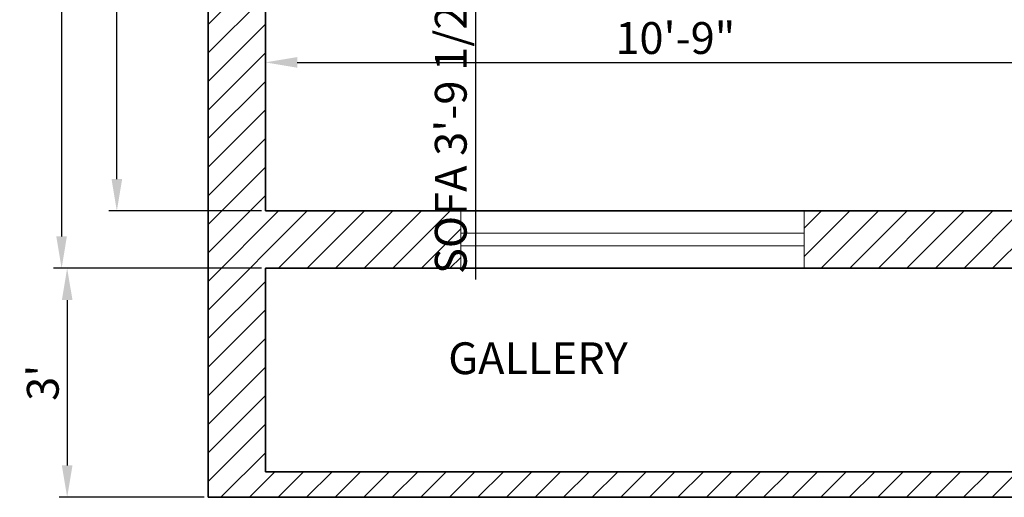
# Model space of a CAD drawing. Units: inches. Extents: x -33 to 381, y -443 to 47.
# Tile 1 of 5: x -33 to 122, y -383 to -308. Entities that reach past the tile are written whole.
import ezdxf

# ---------------------------------------------------------------- set-up
doc = ezdxf.new("R2010")
doc.units = ezdxf.units.IN
for name, color, linetype, lineweight in [('A-ANNO-DIMS', 2, 'Continuous', 18), ('A-AREA-IDEN', 7, 'Continuous', 18), ('A-GLAZ', 4, 'Continuous', 18), ('A-WALL', 7, 'Continuous', 35), ('A-WALL-PATT', 251, 'Continuous', 13)]:
    doc.layers.add(name, color=color, linetype=linetype, lineweight=lineweight)
doc.styles.get("Standard").update_dxf_attribs({"font": 'arial.ttf'})
doc.dimstyles.new('ISO-25', dxfattribs={"dimtxt": 5, "dimasz": 5, "dimexe": 1.25, "dimexo": 0.625, "dimtad": 1, "dimlunit": 3, "dimtxsty": 'Standard', "dimcen": 2.5, "dimadec": 0, "dimazin": 0, "dimtfac": 1, "dimtmove": 0, "dimatfit": 3, "dimfxl": 1, "dimarcsym": 0})
pattern_1 = [(45, (-607.8963, -64.2963), (-2.245064, 2.245064), [])]

# ---------------------------------------------------------------- blocks, each defined once
blk = doc.blocks.new('*D11')
at = {"layer": 'A-ANNO-DIMS', "color": 0, "lineweight": -2, "transparency": 16777216}
for p, q in [((-4.08, 13.18), (-27.74, 13.18)), ((-26.49, 8.18), (-26.49, -341.82)), ((4.92, -346.82), (-27.74, -346.82))]:
    blk.add_line(p, q, dxfattribs=at)
at = {"layer": 'A-ANNO-DIMS', "color": 0, "transparency": 16777216}
for points in [[(-27.33, 8.18), (-25.66, 8.18), (-26.49, 13.18)], [(-27.33, -341.82), (-25.66, -341.82), (-26.49, -346.82)]]:
    blk.add_solid(points, dxfattribs=at)
at = {"layer": 'Defpoints', "color": 0, "transparency": 16777216}
for p in [(-3.46, 13.18), (-26.49, -346.82), (5.54, -346.82)]:
    blk.add_point(p, dxfattribs=at)
at = {"layer": 'A-ANNO-DIMS', "color": 0, "transparency": 16777216, "insert": (-29.67, -166.82), "char_height": 5, "attachment_point": 5, "rotation": 90}
blk.add_mtext("30'", dxfattribs=at)
blk = doc.blocks.new('*D12')
at = {"layer": 'A-ANNO-DIMS', "color": 0, "lineweight": -2, "transparency": 16777216}
for p, q in [((-4.08, -346.82), (-26.87, -346.82)), ((-25.62, -351.82), (-25.62, -377.82)), ((-4.08, -382.82), (-26.87, -382.82))]:
    blk.add_line(p, q, dxfattribs=at)
at = {"layer": 'A-ANNO-DIMS', "color": 0, "transparency": 16777216}
for points in [[(-26.45, -351.82), (-24.78, -351.82), (-25.62, -346.82)], [(-26.45, -377.82), (-24.78, -377.82), (-25.62, -382.82)]]:
    blk.add_solid(points, dxfattribs=at)
at = {"layer": 'Defpoints', "color": 0, "transparency": 16777216}
for p in [(-3.46, -346.82), (-25.62, -382.82), (-3.46, -382.82)]:
    blk.add_point(p, dxfattribs=at)
at = {"layer": 'A-ANNO-DIMS', "color": 0, "transparency": 16777216, "insert": (-28.8, -364.82), "char_height": 5, "attachment_point": 5, "rotation": 90}
blk.add_mtext("3'", dxfattribs=at)
blk = doc.blocks.new('*D21')
at = {"layer": 'A-ANNO-DIMS', "color": 0, "lineweight": -2, "transparency": 16777216}
for p, q in [((32.37, -251.08), (39.8, -251.08)), ((38.55, -256.08), (38.55, -291.45)), ((32.37, -296.45), (39.8, -296.45)), ((38.55, -296.45), (38.55, -348.58))]:
    blk.add_line(p, q, dxfattribs=at)
at = {"layer": 'A-ANNO-DIMS', "color": 0, "transparency": 16777216}
for points in [[(37.71, -256.08), (39.38, -256.08), (38.55, -251.08)], [(37.71, -291.45), (39.38, -291.45), (38.55, -296.45)]]:
    blk.add_solid(points, dxfattribs=at)
at = {"layer": 'Defpoints', "color": 0, "transparency": 16777216}
for p in [(31.74, -251.08), (31.74, -296.45), (38.55, -296.45)]:
    blk.add_point(p, dxfattribs=at)
at = {"layer": 'A-ANNO-DIMS', "color": 0, "transparency": 16777216, "insert": (35.33, -325.02), "char_height": 5, "attachment_point": 5, "rotation": 90}
blk.add_mtext('SOFA 3\'-9 1/2"', dxfattribs=at)
blk = doc.blocks.new('*D45')
at = {"layer": 'A-ANNO-DIMS', "color": 0, "lineweight": -2, "transparency": 16777216}
for p, q in [((4.92, -218.82), (-19.06, -218.82)), ((-17.81, -332.82), (-17.81, -223.82)), ((4.92, -337.82), (-19.06, -337.82))]:
    blk.add_line(p, q, dxfattribs=at)
at = {"layer": 'A-ANNO-DIMS', "color": 0, "transparency": 16777216}
for points in [[(-18.64, -223.82), (-16.98, -223.82), (-17.81, -218.82)], [(-18.64, -332.82), (-16.98, -332.82), (-17.81, -337.82)]]:
    blk.add_solid(points, dxfattribs=at)
at = {"layer": 'Defpoints', "color": 0, "transparency": 16777216}
for p in [(-17.81, -218.82), (5.54, -218.82), (5.54, -337.82)]:
    blk.add_point(p, dxfattribs=at)
at = {"layer": 'A-ANNO-DIMS', "color": 0, "transparency": 16777216, "insert": (-20.99, -278.32), "char_height": 5, "attachment_point": 5, "rotation": 90}
blk.add_mtext('9\'-11"', dxfattribs=at)
blk = doc.blocks.new('*D63')
at = {"layer": 'A-ANNO-DIMS', "color": 0, "lineweight": -2, "transparency": 16777216}
for p, q in [((5.54, -337.2), (5.54, -313.22)), ((134.42, -337.2), (134.42, -313.22)), ((10.54, -314.47), (129.42, -314.47))]:
    blk.add_line(p, q, dxfattribs=at)
at = {"layer": 'A-ANNO-DIMS', "color": 0, "transparency": 16777216}
for points in [[(10.54, -313.64), (10.54, -315.3), (5.54, -314.47)], [(129.42, -313.64), (129.42, -315.3), (134.42, -314.47)]]:
    blk.add_solid(points, dxfattribs=at)
at = {"layer": 'Defpoints', "color": 0, "transparency": 16777216}
for p in [(134.42, -314.47), (5.54, -337.82), (134.42, -337.82)]:
    blk.add_point(p, dxfattribs=at)
at = {"layer": 'A-ANNO-DIMS', "color": 0, "transparency": 16777216, "insert": (69.98, -311.29), "char_height": 5, "attachment_point": 5}
blk.add_mtext('10\'-9"', dxfattribs=at)

msp = doc.modelspace()

# ---------------------------------------------------------------- hatches: boundary and pattern name
at = {"layer": 'A-WALL-PATT'}
h = msp.add_hatch(dxfattribs=at)
h.set_pattern_fill('ANSI31', color=256)
h.set_pattern_definition(pattern_1)
h.paths.add_polyline_path([(356.541, 13.18), (-3.459, 13.18), (-3.459, -346.82), (-3.459, -382.82), (254.541, -382.82), (254.541, -378.82), (5.541, -378.82), (5.541, -346.82), (36.25, -346.82), (36.25, -337.82), (5.541, -337.82), (5.541, 4.18), (125.541, 4.18), (125.541, -123.82), (129.541, -123.82), (129.541, -76.862), (147.541, -76.862), (147.541, -72.862), (129.541, -72.862), (129.541, 4.18), (225.541, 4.18), (225.541, -124.82), (181.541, -124.82), (181.541, -120.82), (177.541, -120.82), (177.541, -128.82), (229.541, -128.82), (229.541, 4.18), (347.541, 4.18), (347.541, -119.82), (329.098, -119.82), (329.098, -128.82), (347.541, -128.82), (347.541, -373.82), (343.541, -373.82), (343.541, -382.82), (356.541, -382.82), (356.541, -346.82)])
h.paths.add_polyline_path([(181.541, -35.82), (188.17, -35.82), (188.17, -31.82), (172.2, -31.82), (172.2, -35.82), (177.541, -35.82), (177.541, -90.82), (181.541, -90.82)], flags=17)
h.paths.add_polyline_path([(225.541, -31.82), (222.17, -31.82), (222.17, -35.82), (225.541, -35.82)], flags=17)
h.paths.add_polyline_path([(138.2, -31.82), (129.541, -31.82), (129.541, -35.82), (138.2, -35.82)], flags=17)
h.paths.add_polyline_path([(89.541, -167.82), (85.541, -167.82), (85.541, -209.82), (5.541, -209.82), (5.541, -218.82), (90.906, -218.82), (90.906, -209.82), (89.541, -209.82)], flags=17)
h.paths.add_polyline_path([(165.541, -209.82), (125.541, -209.82), (121.541, -209.82), (121.541, -218.82), (125.541, -218.82), (125.541, -310.82), (160.374, -310.82), (160.374, -301.82), (129.541, -301.82), (129.541, -218.82), (165.541, -218.82)], flags=17)
h.paths.add_polyline_path([(263.541, -209.82), (254.541, -209.82), (201.541, -209.82), (201.541, -218.82), (254.541, -218.82), (254.541, -301.82), (214.374, -301.82), (214.374, -310.82), (254.541, -310.82), (263.541, -310.82)], flags=17)
h.paths.add_polyline_path([(263.541, -128.82), (275.098, -128.82), (275.098, -119.82), (254.541, -119.82), (254.541, -128.82), (254.541, -165.974), (263.541, -165.974)], flags=17)
h.paths.add_polyline_path([(263.541, -373.82), (254.541, -373.82), (254.541, -382.82), (263.541, -382.82)], flags=17)
h = msp.add_hatch(dxfattribs=at)
h.set_pattern_fill('ANSI31', color=256)
h.set_pattern_definition(pattern_1)
h.paths.add_polyline_path([(134.422, -337.82), (90.25, -337.82), (90.25, -346.82), (134.422, -346.82)])

# ---------------------------------------------------------------- linework, layer by layer
at = {"layer": 'A-GLAZ'}
for p, q in [((36.25, -341.32), (90.25, -341.32)), ((36.25, -343.32), (90.25, -343.32))]:
    msp.add_line(p, q, dxfattribs=at)
msp.add_lwpolyline([(36.25, -337.82), (90.25, -337.82), (90.25, -346.82), (36.25, -346.82)], close=True, dxfattribs=at)
at = {"layer": 'A-WALL'}
for p, q in [((-3.459, -346.82), (-3.459, 13.18)), ((5.541, -337.82), (5.541, 4.18)), ((134.422, -337.82), (5.541, -337.82)), ((-3.459, -346.82), (-3.459, -382.82)), ((5.541, -346.82), (5.541, -378.82)), ((134.422, -346.82), (5.541, -346.82)), ((5.541, -378.82), (254.541, -378.82)), ((-3.459, -382.82), (254.541, -382.82))]:
    msp.add_line(p, q, dxfattribs=at)

# ---------------------------------------------------------------- texts
at = {"layer": 'A-AREA-IDEN', "insert": (34.281, -358.467), "char_height": 5, "attachment_point": 1}
msp.add_mtext_dynamic_manual_height_columns('GALLERY', width=62.04936, gutter_width=12.5, heights=[0], dxfattribs=at)

# ---------------------------------------------------------------- dimensions: what is measured, and where the dimension line sits
at = {"layer": 'A-ANNO-DIMS'}
for base, p1, p2, override, picture, middle in [((-26.493, -346.82), (-3.459, 13.18), (5.541, -346.82), {"dimclrd": 0, "dimclre": 0, "dimclrt": 0}, '*D11', (-29.673, -166.82)), ((-17.809, -218.82), (5.541, -337.82), (5.541, -218.82), {"dimdec": 1, "dimlfac": 1, "dimrnd": 0, "dimzin": 1, "dimdsep": 46, "dimlunit": 4, "dimfrac": 2}, '*D45', (-20.987, -278.32)), ((-25.618, -382.82), (-3.459, -346.82), (-3.459, -382.82), {"dimclrd": 0, "dimclre": 0, "dimclrt": 0}, '*D12', (-28.798, -364.82))]:
    dim = msp.add_linear_dim(base=base, p1=p1, p2=p2, angle=90, dimstyle='ISO-25', override=override, dxfattribs=at)
    dim.commit()
    dim.dimension.update_dxf_attribs({"geometry": picture, "text_midpoint": middle})
dim = msp.add_linear_dim(base=(38.547, -296.453), p1=(31.741, -251.076), p2=(31.741, -296.453), angle=270, text='SOFA <>', dimstyle='ISO-25', override={"dimdec": 1, "dimlfac": 1, "dimrnd": 0, "dimzin": 1, "dimdsep": 46, "dimlunit": 4, "dimfrac": 2}, dxfattribs=at)
dim.commit()
dim.dimension.update_dxf_attribs({"geometry": '*D21', "text_midpoint": (35.334, -325.016)})
dim = msp.add_linear_dim(base=(134.422, -314.47), p1=(5.541, -337.82), p2=(134.422, -337.82), dimstyle='ISO-25', override={"dimdec": 1, "dimlfac": 1, "dimrnd": 0, "dimzin": 1, "dimdsep": 46, "dimlunit": 4, "dimfrac": 2}, dxfattribs=at)
dim.commit()
dim.dimension.update_dxf_attribs({"geometry": '*D63', "text_midpoint": (69.981, -311.292)})

doc.saveas('drawing.dxf')
